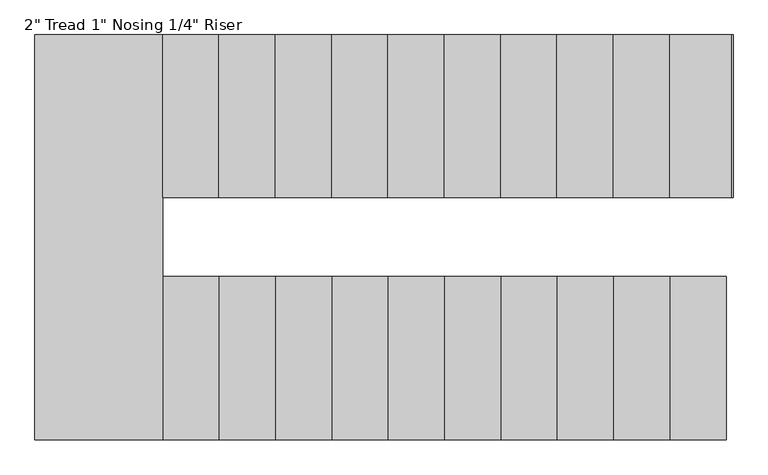
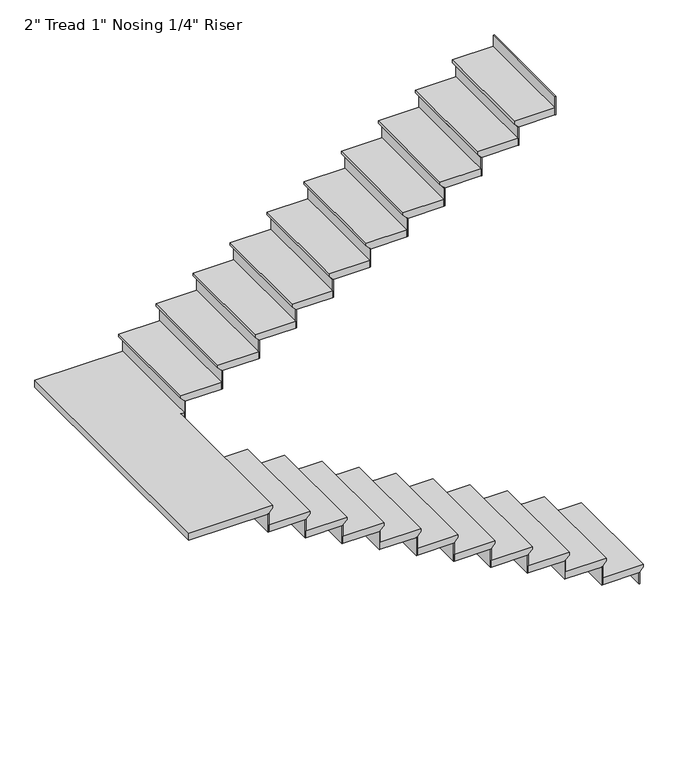
"""IFC4 building model written with IfcOpenShell, lengths in millimetres: stair flight geometry."""

from ifc_helpers import new_model, si_unit, origin, place, context, project, spatial, faceted_brep, source, transform, mapped, element, save


def stair_flight_862ef343(model_context):
    return source(origin(), model_context, "Body", "Brep", [
        faceted_brep([(-3117.2664982, -6914.3822004, 9713.7681818), (-3117.2664982, -6914.3822004, 9732.8181818), (-3117.2664982, -7650.9822004, 9732.8181818), (-3117.2664982, -7650.9822004, 9713.7681818), (-3142.6664982, -6914.3822004, 9688.3681818), (-3142.6664982, -7650.9822004, 9688.3681818), (-3396.6664982, -6914.3822004, 9732.8181818), (-3396.6664982, -7650.9822004, 9732.8181818), (-3142.6664982, -7650.9822004, 9682.0181818), (-3396.6664982, -7650.9822004, 9682.0181818), (-3396.6664982, -6914.3822004, 9682.0181818), (-3142.6664982, -6914.3822004, 9682.0181818)], [[[0, 1, 2, 3]], [[4, 0, 3, 5]], [[2, 1, 6, 7]], [[8, 9, 10, 11]], [[2, 7, 9, 8, 5, 3]], [[8, 11, 4, 5]], [[6, 1, 0, 4, 11, 10]], [[7, 6, 10, 9]]]),
        faceted_brep([(-3142.6664982, -6914.3822004, 9682.0181818), (-3142.6664982, -6914.3822004, 9601.2), (-3149.0164982, -6914.3822004, 9601.2), (-3149.0164982, -6914.3822004, 9682.0181818), (-3142.6664982, -7650.9822004, 9682.0181818), (-3149.0164982, -7650.9822004, 9682.0181818), (-3149.0164982, -7650.9822004, 9601.2), (-3142.6664982, -7650.9822004, 9601.2)], [[[0, 1, 2, 3]], [[4, 5, 6, 7]], [[1, 0, 4, 7]], [[2, 1, 7, 6]], [[3, 2, 6, 5]], [[0, 3, 5, 4]]]),
        faceted_brep([(-3396.6664982, -6914.3822004, 9813.6363636), (-3396.6664982, -6914.3822004, 9682.0181818), (-3403.0164982, -6914.3822004, 9682.0181818), (-3403.0164982, -6914.3822004, 9813.6363636), (-3396.6664982, -7650.9822004, 9813.6363636), (-3403.0164982, -7650.9822004, 9813.6363636), (-3403.0164982, -7650.9822004, 9682.0181818), (-3396.6664982, -7650.9822004, 9682.0181818)], [[[0, 1, 2, 3]], [[4, 5, 6, 7]], [[1, 0, 4, 7]], [[2, 1, 7, 6]], [[3, 2, 6, 5]], [[0, 3, 5, 4]]]),
        faceted_brep([(-3371.2664982, -7650.9822004, 9864.4363636), (-3371.2664982, -6914.3822004, 9864.4363636), (-3650.6664982, -6914.3822004, 9864.4363636), (-3650.6664982, -7650.9822004, 9864.4363636), (-3396.6664982, -7650.9822004, 9813.6363636), (-3650.6664982, -7650.9822004, 9813.6363636), (-3650.6664982, -6914.3822004, 9813.6363636), (-3396.6664982, -6914.3822004, 9813.6363636), (-3396.6664982, -7650.9822004, 9819.9863636), (-3371.2664982, -7650.9822004, 9845.3863636), (-3396.6664982, -6914.3822004, 9819.9863636), (-3371.2664982, -6914.3822004, 9845.3863636)], [[[0, 1, 2, 3]], [[4, 5, 6, 7]], [[0, 3, 5, 4, 8, 9]], [[4, 7, 10, 8]], [[2, 1, 11, 10, 7, 6]], [[3, 2, 6, 5]], [[11, 1, 0, 9]], [[10, 11, 9, 8]]]),
        faceted_brep([(-3650.6664982, -6914.3822004, 9945.2545455), (-3650.6664982, -6914.3822004, 9813.6363636), (-3657.0164982, -6914.3822004, 9813.6363636), (-3657.0164982, -6914.3822004, 9945.2545455), (-3650.6664982, -7650.9822004, 9945.2545455), (-3657.0164982, -7650.9822004, 9945.2545455), (-3657.0164982, -7650.9822004, 9813.6363636), (-3650.6664982, -7650.9822004, 9813.6363636)], [[[0, 1, 2, 3]], [[4, 5, 6, 7]], [[1, 0, 4, 7]], [[2, 1, 7, 6]], [[3, 2, 6, 5]], [[0, 3, 5, 4]]]),
        faceted_brep([(-3625.2664982, -7650.9822004, 9996.0545455), (-3625.2664982, -6914.3822004, 9996.0545455), (-3904.6664982, -6914.3822004, 9996.0545455), (-3904.6664982, -7650.9822004, 9996.0545455), (-3650.6664982, -7650.9822004, 9945.2545455), (-3904.6664982, -7650.9822004, 9945.2545455), (-3904.6664982, -6914.3822004, 9945.2545455), (-3650.6664982, -6914.3822004, 9945.2545455), (-3650.6664982, -7650.9822004, 9951.6045455), (-3625.2664982, -7650.9822004, 9977.0045455), (-3650.6664982, -6914.3822004, 9951.6045455), (-3625.2664982, -6914.3822004, 9977.0045455)], [[[0, 1, 2, 3]], [[4, 5, 6, 7]], [[0, 3, 5, 4, 8, 9]], [[4, 7, 10, 8]], [[2, 1, 11, 10, 7, 6]], [[3, 2, 6, 5]], [[11, 1, 0, 9]], [[10, 11, 9, 8]]]),
        faceted_brep([(-3904.6664982, -6914.3822004, 10076.8727273), (-3904.6664982, -6914.3822004, 9945.2545455), (-3911.0164982, -6914.3822004, 9945.2545455), (-3911.0164982, -6914.3822004, 10076.8727273), (-3904.6664982, -7650.9822004, 10076.8727273), (-3911.0164982, -7650.9822004, 10076.8727273), (-3911.0164982, -7650.9822004, 9945.2545455), (-3904.6664982, -7650.9822004, 9945.2545455)], [[[0, 1, 2, 3]], [[4, 5, 6, 7]], [[1, 0, 4, 7]], [[2, 1, 7, 6]], [[3, 2, 6, 5]], [[0, 3, 5, 4]]]),
        faceted_brep([(-3879.2664982, -7650.9822004, 10127.6727273), (-3879.2664982, -6914.3822004, 10127.6727273), (-4158.6664982, -6914.3822004, 10127.6727273), (-4158.6664982, -7650.9822004, 10127.6727273), (-3904.6664982, -7650.9822004, 10076.8727273), (-4158.6664982, -7650.9822004, 10076.8727273), (-4158.6664982, -6914.3822004, 10076.8727273), (-3904.6664982, -6914.3822004, 10076.8727273), (-3904.6664982, -7650.9822004, 10083.2227273), (-3879.2664982, -7650.9822004, 10108.6227273), (-3904.6664982, -6914.3822004, 10083.2227273), (-3879.2664982, -6914.3822004, 10108.6227273)], [[[0, 1, 2, 3]], [[4, 5, 6, 7]], [[0, 3, 5, 4, 8, 9]], [[4, 7, 10, 8]], [[2, 1, 11, 10, 7, 6]], [[3, 2, 6, 5]], [[11, 1, 0, 9]], [[10, 11, 9, 8]]]),
        faceted_brep([(-4158.6664982, -6914.3822004, 10208.4909091), (-4158.6664982, -6914.3822004, 10076.8727273), (-4165.0164982, -6914.3822004, 10076.8727273), (-4165.0164982, -6914.3822004, 10208.4909091), (-4158.6664982, -7650.9822004, 10208.4909091), (-4165.0164982, -7650.9822004, 10208.4909091), (-4165.0164982, -7650.9822004, 10076.8727273), (-4158.6664982, -7650.9822004, 10076.8727273)], [[[0, 1, 2, 3]], [[4, 5, 6, 7]], [[1, 0, 4, 7]], [[2, 1, 7, 6]], [[3, 2, 6, 5]], [[0, 3, 5, 4]]]),
        faceted_brep([(-4133.2664982, -7650.9822004, 10259.2909091), (-4133.2664982, -6914.3822004, 10259.2909091), (-4412.6664982, -6914.3822004, 10259.2909091), (-4412.6664982, -7650.9822004, 10259.2909091), (-4158.6664982, -7650.9822004, 10208.4909091), (-4412.6664982, -7650.9822004, 10208.4909091), (-4412.6664982, -6914.3822004, 10208.4909091), (-4158.6664982, -6914.3822004, 10208.4909091), (-4158.6664982, -7650.9822004, 10214.8409091), (-4133.2664982, -7650.9822004, 10240.2409091), (-4158.6664982, -6914.3822004, 10214.8409091), (-4133.2664982, -6914.3822004, 10240.2409091)], [[[0, 1, 2, 3]], [[4, 5, 6, 7]], [[0, 3, 5, 4, 8, 9]], [[4, 7, 10, 8]], [[2, 1, 11, 10, 7, 6]], [[3, 2, 6, 5]], [[11, 1, 0, 9]], [[10, 11, 9, 8]]]),
        faceted_brep([(-4412.6664982, -6914.3822004, 10340.1090909), (-4412.6664982, -6914.3822004, 10208.4909091), (-4419.0164982, -6914.3822004, 10208.4909091), (-4419.0164982, -6914.3822004, 10340.1090909), (-4412.6664982, -7650.9822004, 10340.1090909), (-4419.0164982, -7650.9822004, 10340.1090909), (-4419.0164982, -7650.9822004, 10208.4909091), (-4412.6664982, -7650.9822004, 10208.4909091)], [[[0, 1, 2, 3]], [[4, 5, 6, 7]], [[1, 0, 4, 7]], [[2, 1, 7, 6]], [[3, 2, 6, 5]], [[0, 3, 5, 4]]]),
        faceted_brep([(-4387.2664982, -7650.9822004, 10390.9090909), (-4387.2664982, -6914.3822004, 10390.9090909), (-4666.6664982, -6914.3822004, 10390.9090909), (-4666.6664982, -7650.9822004, 10390.9090909), (-4412.6664982, -7650.9822004, 10340.1090909), (-4666.6664982, -7650.9822004, 10340.1090909), (-4666.6664982, -6914.3822004, 10340.1090909), (-4412.6664982, -6914.3822004, 10340.1090909), (-4412.6664982, -7650.9822004, 10346.4590909), (-4387.2664982, -7650.9822004, 10371.8590909), (-4412.6664982, -6914.3822004, 10346.4590909), (-4387.2664982, -6914.3822004, 10371.8590909)], [[[0, 1, 2, 3]], [[4, 5, 6, 7]], [[0, 3, 5, 4, 8, 9]], [[4, 7, 10, 8]], [[2, 1, 11, 10, 7, 6]], [[3, 2, 6, 5]], [[11, 1, 0, 9]], [[10, 11, 9, 8]]]),
        faceted_brep([(-4666.6664982, -6914.3822004, 10471.7272727), (-4666.6664982, -6914.3822004, 10340.1090909), (-4673.0164982, -6914.3822004, 10340.1090909), (-4673.0164982, -6914.3822004, 10471.7272727), (-4666.6664982, -7650.9822004, 10471.7272727), (-4673.0164982, -7650.9822004, 10471.7272727), (-4673.0164982, -7650.9822004, 10340.1090909), (-4666.6664982, -7650.9822004, 10340.1090909)], [[[0, 1, 2, 3]], [[4, 5, 6, 7]], [[1, 0, 4, 7]], [[2, 1, 7, 6]], [[3, 2, 6, 5]], [[0, 3, 5, 4]]]),
        faceted_brep([(-4641.2664982, -7650.9822004, 10522.5272727), (-4641.2664982, -6914.3822004, 10522.5272727), (-4920.6664982, -6914.3822004, 10522.5272727), (-4920.6664982, -7650.9822004, 10522.5272727), (-4666.6664982, -7650.9822004, 10471.7272727), (-4920.6664982, -7650.9822004, 10471.7272727), (-4920.6664982, -6914.3822004, 10471.7272727), (-4666.6664982, -6914.3822004, 10471.7272727), (-4666.6664982, -7650.9822004, 10478.0772727), (-4641.2664982, -7650.9822004, 10503.4772727), (-4666.6664982, -6914.3822004, 10478.0772727), (-4641.2664982, -6914.3822004, 10503.4772727)], [[[0, 1, 2, 3]], [[4, 5, 6, 7]], [[0, 3, 5, 4, 8, 9]], [[4, 7, 10, 8]], [[2, 1, 11, 10, 7, 6]], [[3, 2, 6, 5]], [[11, 1, 0, 9]], [[10, 11, 9, 8]]]),
        faceted_brep([(-4920.6664982, -6914.3822004, 10603.3454545), (-4920.6664982, -6914.3822004, 10471.7272727), (-4927.0164982, -6914.3822004, 10471.7272727), (-4927.0164982, -6914.3822004, 10603.3454545), (-4920.6664982, -7650.9822004, 10603.3454545), (-4927.0164982, -7650.9822004, 10603.3454545), (-4927.0164982, -7650.9822004, 10471.7272727), (-4920.6664982, -7650.9822004, 10471.7272727)], [[[0, 1, 2, 3]], [[4, 5, 6, 7]], [[1, 0, 4, 7]], [[2, 1, 7, 6]], [[3, 2, 6, 5]], [[0, 3, 5, 4]]]),
        faceted_brep([(-4895.2664982, -7650.9822004, 10654.1454545), (-4895.2664982, -6914.3822004, 10654.1454545), (-5174.6664982, -6914.3822004, 10654.1454545), (-5174.6664982, -7650.9822004, 10654.1454545), (-4920.6664982, -7650.9822004, 10603.3454545), (-5174.6664982, -7650.9822004, 10603.3454545), (-5174.6664982, -6914.3822004, 10603.3454545), (-4920.6664982, -6914.3822004, 10603.3454545), (-4920.6664982, -7650.9822004, 10609.6954545), (-4895.2664982, -7650.9822004, 10635.0954545), (-4920.6664982, -6914.3822004, 10609.6954545), (-4895.2664982, -6914.3822004, 10635.0954545)], [[[0, 1, 2, 3]], [[4, 5, 6, 7]], [[0, 3, 5, 4, 8, 9]], [[4, 7, 10, 8]], [[2, 1, 11, 10, 7, 6]], [[3, 2, 6, 5]], [[11, 1, 0, 9]], [[10, 11, 9, 8]]]),
        faceted_brep([(-5174.6664982, -6914.3822004, 10734.9636364), (-5174.6664982, -6914.3822004, 10603.3454545), (-5181.0164982, -6914.3822004, 10603.3454545), (-5181.0164982, -6914.3822004, 10734.9636364), (-5174.6664982, -7650.9822004, 10734.9636364), (-5181.0164982, -7650.9822004, 10734.9636364), (-5181.0164982, -7650.9822004, 10603.3454545), (-5174.6664982, -7650.9822004, 10603.3454545)], [[[0, 1, 2, 3]], [[4, 5, 6, 7]], [[1, 0, 4, 7]], [[2, 1, 7, 6]], [[3, 2, 6, 5]], [[0, 3, 5, 4]]]),
        faceted_brep([(-5149.2664982, -7650.9822004, 10785.7636364), (-5149.2664982, -6914.3822004, 10785.7636364), (-5428.6664982, -6914.3822004, 10785.7636364), (-5428.6664982, -7650.9822004, 10785.7636364), (-5174.6664982, -7650.9822004, 10734.9636364), (-5428.6664982, -7650.9822004, 10734.9636364), (-5428.6664982, -6914.3822004, 10734.9636364), (-5174.6664982, -6914.3822004, 10734.9636364), (-5174.6664982, -7650.9822004, 10741.3136364), (-5149.2664982, -7650.9822004, 10766.7136364), (-5174.6664982, -6914.3822004, 10741.3136364), (-5149.2664982, -6914.3822004, 10766.7136364)], [[[0, 1, 2, 3]], [[4, 5, 6, 7]], [[0, 3, 5, 4, 8, 9]], [[4, 7, 10, 8]], [[2, 1, 11, 10, 7, 6]], [[3, 2, 6, 5]], [[11, 1, 0, 9]], [[10, 11, 9, 8]]]),
        faceted_brep([(-5428.6664982, -6914.3822004, 10866.5818182), (-5428.6664982, -6914.3822004, 10734.9636364), (-5435.0164982, -6914.3822004, 10734.9636364), (-5435.0164982, -6914.3822004, 10866.5818182), (-5428.6664982, -7650.9822004, 10866.5818182), (-5435.0164982, -7650.9822004, 10866.5818182), (-5435.0164982, -7650.9822004, 10734.9636364), (-5428.6664982, -7650.9822004, 10734.9636364)], [[[0, 1, 2, 3]], [[4, 5, 6, 7]], [[1, 0, 4, 7]], [[2, 1, 7, 6]], [[3, 2, 6, 5]], [[0, 3, 5, 4]]]),
        faceted_brep([(-5403.2664982, -7650.9822004, 10917.3818182), (-5403.2664982, -6914.3822004, 10917.3818182), (-5682.6664982, -6914.3822004, 10917.3818182), (-5682.6664982, -7650.9822004, 10917.3818182), (-5428.6664982, -7650.9822004, 10866.5818182), (-5682.6664982, -7650.9822004, 10866.5818182), (-5682.6664982, -6914.3822004, 10866.5818182), (-5428.6664982, -6914.3822004, 10866.5818182), (-5428.6664982, -7650.9822004, 10872.9318182), (-5403.2664982, -7650.9822004, 10898.3318182), (-5428.6664982, -6914.3822004, 10872.9318182), (-5403.2664982, -6914.3822004, 10898.3318182)], [[[0, 1, 2, 3]], [[4, 5, 6, 7]], [[0, 3, 5, 4, 8, 9]], [[4, 7, 10, 8]], [[2, 1, 11, 10, 7, 6]], [[3, 2, 6, 5]], [[11, 1, 0, 9]], [[10, 11, 9, 8]]]),
        faceted_brep([(-5682.6664982, -6914.3822004, 10998.2), (-5682.6664982, -6914.3822004, 10866.5818182), (-5689.0164982, -6914.3822004, 10866.5818182), (-5689.0164982, -6914.3822004, 10998.2), (-5682.6664982, -7650.9822004, 10998.2), (-5689.0164982, -7650.9822004, 10998.2), (-5689.0164982, -7650.9822004, 10866.5818182), (-5682.6664982, -7650.9822004, 10866.5818182)], [[[0, 1, 2, 3]], [[4, 5, 6, 7]], [[1, 0, 4, 7]], [[2, 1, 7, 6]], [[3, 2, 6, 5]], [[0, 3, 5, 4]]]),
        faceted_brep([(-5631.8664982, -5824.7082131, 11049.0), (-6232.5131972, -5824.7082131, 11049.0), (-6232.5131972, -7650.9822004, 11049.0), (-5657.2664982, -7650.9822004, 11049.0), (-5657.2664982, -6558.7822004, 11049.0), (-5631.8664982, -6558.7822004, 11049.0), (-6232.5131972, -5824.7082131, 10998.2), (-5631.8664982, -5824.7082131, 10998.2), (-5631.8664982, -6558.7822004, 10998.2), (-5657.2664982, -6558.7822004, 10998.2), (-5657.2664982, -6914.3822004, 10998.2), (-5682.6664982, -6914.3822004, 10998.2), (-5682.6664982, -7650.9822004, 10998.2), (-6232.5131972, -7650.9822004, 10998.2), (-5682.6664982, -6914.3822004, 11004.55), (-5682.6664982, -7650.9822004, 11004.55), (-5657.2664982, -7650.9822004, 11029.95), (-5657.2664982, -6914.3822004, 11029.95)], [[[0, 1, 2, 3, 4, 5]], [[6, 7, 8, 9, 10, 11, 12, 13]], [[1, 0, 7, 6]], [[2, 1, 6, 13]], [[12, 11, 14, 15]], [[4, 3, 16, 17, 10, 9]], [[5, 4, 9, 8]], [[0, 5, 8, 7]], [[16, 15, 14, 17]], [[3, 2, 13, 12, 15, 16]], [[11, 10, 17, 14]]]),
        faceted_brep([(-5631.8664982, -6558.7822004, 11129.8181818), (-5631.8664982, -6558.7822004, 10998.2), (-5625.5164982, -6558.7822004, 10998.2), (-5625.5164982, -6558.7822004, 11129.8181818), (-5631.8664982, -5824.7082131, 11129.8181818), (-5625.5164982, -5824.7082131, 11129.8181818), (-5625.5164982, -5824.7082131, 10998.2), (-5631.8664982, -5824.7082131, 10998.2)], [[[0, 1, 2, 3]], [[4, 5, 6, 7]], [[1, 0, 4, 7]], [[2, 1, 7, 6]], [[3, 2, 6, 5]], [[0, 3, 5, 4]]]),
        faceted_brep([(-5657.2664982, -5824.7082131, 11180.6181818), (-5657.2664982, -6558.7822004, 11180.6181818), (-5377.8664982, -6558.7822004, 11180.6181818), (-5377.8664982, -5824.7082131, 11180.6181818), (-5631.8664982, -5824.7082131, 11129.8181818), (-5377.8664982, -5824.7082131, 11129.8181818), (-5377.8664982, -6558.7822004, 11129.8181818), (-5631.8664982, -6558.7822004, 11129.8181818), (-5631.8664982, -5824.7082131, 11136.1681818), (-5657.2664982, -5824.7082131, 11161.5681818), (-5631.8664982, -6558.7822004, 11136.1681818), (-5657.2664982, -6558.7822004, 11161.5681818)], [[[0, 1, 2, 3]], [[4, 5, 6, 7]], [[0, 3, 5, 4, 8, 9]], [[4, 7, 10, 8]], [[2, 1, 11, 10, 7, 6]], [[3, 2, 6, 5]], [[11, 1, 0, 9]], [[10, 11, 9, 8]]]),
        faceted_brep([(-5377.8664982, -6558.7822004, 11261.4363636), (-5377.8664982, -6558.7822004, 11129.8181818), (-5371.5164982, -6558.7822004, 11129.8181818), (-5371.5164982, -6558.7822004, 11261.4363636), (-5377.8664982, -5824.7082131, 11261.4363636), (-5371.5164982, -5824.7082131, 11261.4363636), (-5371.5164982, -5824.7082131, 11129.8181818), (-5377.8664982, -5824.7082131, 11129.8181818)], [[[0, 1, 2, 3]], [[4, 5, 6, 7]], [[1, 0, 4, 7]], [[2, 1, 7, 6]], [[3, 2, 6, 5]], [[0, 3, 5, 4]]]),
        faceted_brep([(-5403.2664982, -5824.7082131, 11312.2363636), (-5403.2664982, -6558.7822004, 11312.2363636), (-5123.8664982, -6558.7822004, 11312.2363636), (-5123.8664982, -5824.7082131, 11312.2363636), (-5377.8664982, -5824.7082131, 11261.4363636), (-5123.8664982, -5824.7082131, 11261.4363636), (-5123.8664982, -6558.7822004, 11261.4363636), (-5377.8664982, -6558.7822004, 11261.4363636), (-5377.8664982, -5824.7082131, 11267.7863636), (-5403.2664982, -5824.7082131, 11293.1863636), (-5377.8664982, -6558.7822004, 11267.7863636), (-5403.2664982, -6558.7822004, 11293.1863636)], [[[0, 1, 2, 3]], [[4, 5, 6, 7]], [[0, 3, 5, 4, 8, 9]], [[4, 7, 10, 8]], [[2, 1, 11, 10, 7, 6]], [[3, 2, 6, 5]], [[11, 1, 0, 9]], [[10, 11, 9, 8]]]),
        faceted_brep([(-5123.8664982, -6558.7822004, 11393.0545455), (-5123.8664982, -6558.7822004, 11261.4363636), (-5117.5164982, -6558.7822004, 11261.4363636), (-5117.5164982, -6558.7822004, 11393.0545455), (-5123.8664982, -5824.7082131, 11393.0545455), (-5117.5164982, -5824.7082131, 11393.0545455), (-5117.5164982, -5824.7082131, 11261.4363636), (-5123.8664982, -5824.7082131, 11261.4363636)], [[[0, 1, 2, 3]], [[4, 5, 6, 7]], [[1, 0, 4, 7]], [[2, 1, 7, 6]], [[3, 2, 6, 5]], [[0, 3, 5, 4]]]),
        faceted_brep([(-5149.2664982, -5824.7082131, 11443.8545455), (-5149.2664982, -6558.7822004, 11443.8545455), (-4869.8664982, -6558.7822004, 11443.8545455), (-4869.8664982, -5824.7082131, 11443.8545455), (-5123.8664982, -5824.7082131, 11393.0545455), (-4869.8664982, -5824.7082131, 11393.0545455), (-4869.8664982, -6558.7822004, 11393.0545455), (-5123.8664982, -6558.7822004, 11393.0545455), (-5123.8664982, -5824.7082131, 11399.4045455), (-5149.2664982, -5824.7082131, 11424.8045455), (-5123.8664982, -6558.7822004, 11399.4045455), (-5149.2664982, -6558.7822004, 11424.8045455)], [[[0, 1, 2, 3]], [[4, 5, 6, 7]], [[0, 3, 5, 4, 8, 9]], [[4, 7, 10, 8]], [[2, 1, 11, 10, 7, 6]], [[3, 2, 6, 5]], [[11, 1, 0, 9]], [[10, 11, 9, 8]]]),
        faceted_brep([(-4869.8664982, -6558.7822004, 11524.6727273), (-4869.8664982, -6558.7822004, 11393.0545455), (-4863.5164982, -6558.7822004, 11393.0545455), (-4863.5164982, -6558.7822004, 11524.6727273), (-4869.8664982, -5824.7082131, 11524.6727273), (-4863.5164982, -5824.7082131, 11524.6727273), (-4863.5164982, -5824.7082131, 11393.0545455), (-4869.8664982, -5824.7082131, 11393.0545455)], [[[0, 1, 2, 3]], [[4, 5, 6, 7]], [[1, 0, 4, 7]], [[2, 1, 7, 6]], [[3, 2, 6, 5]], [[0, 3, 5, 4]]]),
        faceted_brep([(-4895.2664982, -5824.7082131, 11575.4727273), (-4895.2664982, -6558.7822004, 11575.4727273), (-4615.8664982, -6558.7822004, 11575.4727273), (-4615.8664982, -5824.7082131, 11575.4727273), (-4869.8664982, -5824.7082131, 11524.6727273), (-4615.8664982, -5824.7082131, 11524.6727273), (-4615.8664982, -6558.7822004, 11524.6727273), (-4869.8664982, -6558.7822004, 11524.6727273), (-4869.8664982, -5824.7082131, 11531.0227273), (-4895.2664982, -5824.7082131, 11556.4227273), (-4869.8664982, -6558.7822004, 11531.0227273), (-4895.2664982, -6558.7822004, 11556.4227273)], [[[0, 1, 2, 3]], [[4, 5, 6, 7]], [[0, 3, 5, 4, 8, 9]], [[4, 7, 10, 8]], [[2, 1, 11, 10, 7, 6]], [[3, 2, 6, 5]], [[11, 1, 0, 9]], [[10, 11, 9, 8]]]),
        faceted_brep([(-4615.8664982, -6558.7822004, 11656.2909091), (-4615.8664982, -6558.7822004, 11524.6727273), (-4609.5164982, -6558.7822004, 11524.6727273), (-4609.5164982, -6558.7822004, 11656.2909091), (-4615.8664982, -5824.7082131, 11656.2909091), (-4609.5164982, -5824.7082131, 11656.2909091), (-4609.5164982, -5824.7082131, 11524.6727273), (-4615.8664982, -5824.7082131, 11524.6727273)], [[[0, 1, 2, 3]], [[4, 5, 6, 7]], [[1, 0, 4, 7]], [[2, 1, 7, 6]], [[3, 2, 6, 5]], [[0, 3, 5, 4]]]),
        faceted_brep([(-4641.2664982, -5824.7082131, 11707.0909091), (-4641.2664982, -6558.7822004, 11707.0909091), (-4361.8664982, -6558.7822004, 11707.0909091), (-4361.8664982, -5824.7082131, 11707.0909091), (-4615.8664982, -5824.7082131, 11656.2909091), (-4361.8664982, -5824.7082131, 11656.2909091), (-4361.8664982, -6558.7822004, 11656.2909091), (-4615.8664982, -6558.7822004, 11656.2909091), (-4615.8664982, -5824.7082131, 11662.6409091), (-4641.2664982, -5824.7082131, 11688.0409091), (-4615.8664982, -6558.7822004, 11662.6409091), (-4641.2664982, -6558.7822004, 11688.0409091)], [[[0, 1, 2, 3]], [[4, 5, 6, 7]], [[0, 3, 5, 4, 8, 9]], [[4, 7, 10, 8]], [[2, 1, 11, 10, 7, 6]], [[3, 2, 6, 5]], [[11, 1, 0, 9]], [[10, 11, 9, 8]]]),
        faceted_brep([(-4361.8664982, -6558.7822004, 11787.9090909), (-4361.8664982, -6558.7822004, 11656.2909091), (-4355.5164982, -6558.7822004, 11656.2909091), (-4355.5164982, -6558.7822004, 11787.9090909), (-4361.8664982, -5824.7082131, 11787.9090909), (-4355.5164982, -5824.7082131, 11787.9090909), (-4355.5164982, -5824.7082131, 11656.2909091), (-4361.8664982, -5824.7082131, 11656.2909091)], [[[0, 1, 2, 3]], [[4, 5, 6, 7]], [[1, 0, 4, 7]], [[2, 1, 7, 6]], [[3, 2, 6, 5]], [[0, 3, 5, 4]]]),
        faceted_brep([(-4387.2664982, -5824.7082131, 11838.7090909), (-4387.2664982, -6558.7822004, 11838.7090909), (-4107.8664982, -6558.7822004, 11838.7090909), (-4107.8664982, -5824.7082131, 11838.7090909), (-4361.8664982, -5824.7082131, 11787.9090909), (-4107.8664982, -5824.7082131, 11787.9090909), (-4107.8664982, -6558.7822004, 11787.9090909), (-4361.8664982, -6558.7822004, 11787.9090909), (-4361.8664982, -5824.7082131, 11794.2590909), (-4387.2664982, -5824.7082131, 11819.6590909), (-4361.8664982, -6558.7822004, 11794.2590909), (-4387.2664982, -6558.7822004, 11819.6590909)], [[[0, 1, 2, 3]], [[4, 5, 6, 7]], [[0, 3, 5, 4, 8, 9]], [[4, 7, 10, 8]], [[2, 1, 11, 10, 7, 6]], [[3, 2, 6, 5]], [[11, 1, 0, 9]], [[10, 11, 9, 8]]]),
        faceted_brep([(-4107.8664982, -6558.7822004, 11919.5272727), (-4107.8664982, -6558.7822004, 11787.9090909), (-4101.5164982, -6558.7822004, 11787.9090909), (-4101.5164982, -6558.7822004, 11919.5272727), (-4107.8664982, -5824.7082131, 11919.5272727), (-4101.5164982, -5824.7082131, 11919.5272727), (-4101.5164982, -5824.7082131, 11787.9090909), (-4107.8664982, -5824.7082131, 11787.9090909)], [[[0, 1, 2, 3]], [[4, 5, 6, 7]], [[1, 0, 4, 7]], [[2, 1, 7, 6]], [[3, 2, 6, 5]], [[0, 3, 5, 4]]]),
        faceted_brep([(-4133.2664982, -5824.7082131, 11970.3272727), (-4133.2664982, -6558.7822004, 11970.3272727), (-3853.8664982, -6558.7822004, 11970.3272727), (-3853.8664982, -5824.7082131, 11970.3272727), (-4107.8664982, -5824.7082131, 11919.5272727), (-3853.8664982, -5824.7082131, 11919.5272727), (-3853.8664982, -6558.7822004, 11919.5272727), (-4107.8664982, -6558.7822004, 11919.5272727), (-4107.8664982, -5824.7082131, 11925.8772727), (-4133.2664982, -5824.7082131, 11951.2772727), (-4107.8664982, -6558.7822004, 11925.8772727), (-4133.2664982, -6558.7822004, 11951.2772727)], [[[0, 1, 2, 3]], [[4, 5, 6, 7]], [[0, 3, 5, 4, 8, 9]], [[4, 7, 10, 8]], [[2, 1, 11, 10, 7, 6]], [[3, 2, 6, 5]], [[11, 1, 0, 9]], [[10, 11, 9, 8]]]),
        faceted_brep([(-3853.8664982, -6558.7822004, 12051.1454545), (-3853.8664982, -6558.7822004, 11919.5272727), (-3847.5164982, -6558.7822004, 11919.5272727), (-3847.5164982, -6558.7822004, 12051.1454545), (-3853.8664982, -5824.7082131, 12051.1454545), (-3847.5164982, -5824.7082131, 12051.1454545), (-3847.5164982, -5824.7082131, 11919.5272727), (-3853.8664982, -5824.7082131, 11919.5272727)], [[[0, 1, 2, 3]], [[4, 5, 6, 7]], [[1, 0, 4, 7]], [[2, 1, 7, 6]], [[3, 2, 6, 5]], [[0, 3, 5, 4]]]),
        faceted_brep([(-3879.2664982, -5824.7082131, 12101.9454545), (-3879.2664982, -6558.7822004, 12101.9454545), (-3599.8664982, -6558.7822004, 12101.9454545), (-3599.8664982, -5824.7082131, 12101.9454545), (-3853.8664982, -5824.7082131, 12051.1454545), (-3599.8664982, -5824.7082131, 12051.1454545), (-3599.8664982, -6558.7822004, 12051.1454545), (-3853.8664982, -6558.7822004, 12051.1454545), (-3853.8664982, -5824.7082131, 12057.4954545), (-3879.2664982, -5824.7082131, 12082.8954545), (-3853.8664982, -6558.7822004, 12057.4954545), (-3879.2664982, -6558.7822004, 12082.8954545)], [[[0, 1, 2, 3]], [[4, 5, 6, 7]], [[0, 3, 5, 4, 8, 9]], [[4, 7, 10, 8]], [[2, 1, 11, 10, 7, 6]], [[3, 2, 6, 5]], [[11, 1, 0, 9]], [[10, 11, 9, 8]]]),
        faceted_brep([(-3599.8664982, -6558.7822004, 12182.7636364), (-3599.8664982, -6558.7822004, 12051.1454545), (-3593.5164982, -6558.7822004, 12051.1454545), (-3593.5164982, -6558.7822004, 12182.7636364), (-3599.8664982, -5824.7082131, 12182.7636364), (-3593.5164982, -5824.7082131, 12182.7636364), (-3593.5164982, -5824.7082131, 12051.1454545), (-3599.8664982, -5824.7082131, 12051.1454545)], [[[0, 1, 2, 3]], [[4, 5, 6, 7]], [[1, 0, 4, 7]], [[2, 1, 7, 6]], [[3, 2, 6, 5]], [[0, 3, 5, 4]]]),
        faceted_brep([(-3625.2664982, -5824.7082131, 12233.5636364), (-3625.2664982, -6558.7822004, 12233.5636364), (-3345.8664982, -6558.7822004, 12233.5636364), (-3345.8664982, -5824.7082131, 12233.5636364), (-3599.8664982, -5824.7082131, 12182.7636364), (-3345.8664982, -5824.7082131, 12182.7636364), (-3345.8664982, -6558.7822004, 12182.7636364), (-3599.8664982, -6558.7822004, 12182.7636364), (-3599.8664982, -5824.7082131, 12189.1136364), (-3625.2664982, -5824.7082131, 12214.5136364), (-3599.8664982, -6558.7822004, 12189.1136364), (-3625.2664982, -6558.7822004, 12214.5136364)], [[[0, 1, 2, 3]], [[4, 5, 6, 7]], [[0, 3, 5, 4, 8, 9]], [[4, 7, 10, 8]], [[2, 1, 11, 10, 7, 6]], [[3, 2, 6, 5]], [[11, 1, 0, 9]], [[10, 11, 9, 8]]]),
        faceted_brep([(-3345.8664982, -6558.7822004, 12314.3818182), (-3345.8664982, -6558.7822004, 12182.7636364), (-3339.5164982, -6558.7822004, 12182.7636364), (-3339.5164982, -6558.7822004, 12314.3818182), (-3345.8664982, -5824.7082131, 12314.3818182), (-3339.5164982, -5824.7082131, 12314.3818182), (-3339.5164982, -5824.7082131, 12182.7636364), (-3345.8664982, -5824.7082131, 12182.7636364)], [[[0, 1, 2, 3]], [[4, 5, 6, 7]], [[1, 0, 4, 7]], [[2, 1, 7, 6]], [[3, 2, 6, 5]], [[0, 3, 5, 4]]]),
        faceted_brep([(-3091.8664982, -6558.7822004, 12446.0), (-3091.8664982, -6558.7822004, 12314.3818182), (-3085.5164982, -6558.7822004, 12314.3818182), (-3085.5164982, -6558.7822004, 12446.0), (-3091.8664982, -5824.7082131, 12446.0), (-3085.5164982, -5824.7082131, 12446.0), (-3085.5164982, -5824.7082131, 12314.3818182), (-3091.8664982, -5824.7082131, 12314.3818182)], [[[0, 1, 2, 3]], [[4, 5, 6, 7]], [[1, 0, 4, 7]], [[2, 1, 7, 6]], [[3, 2, 6, 5]], [[0, 3, 5, 4]]]),
        faceted_brep([(-3371.2664982, -5824.7082131, 12365.1818182), (-3371.2664982, -6558.7822004, 12365.1818182), (-3091.8664982, -6558.7822004, 12365.1818182), (-3091.8664982, -5824.7082131, 12365.1818182), (-3345.8664982, -5824.7082131, 12314.3818182), (-3091.8664982, -5824.7082131, 12314.3818182), (-3091.8664982, -6558.7822004, 12314.3818182), (-3345.8664982, -6558.7822004, 12314.3818182), (-3345.8664982, -5824.7082131, 12320.7318182), (-3371.2664982, -5824.7082131, 12346.1318182), (-3345.8664982, -6558.7822004, 12320.7318182), (-3371.2664982, -6558.7822004, 12346.1318182)], [[[0, 1, 2, 3]], [[4, 5, 6, 7]], [[0, 3, 5, 4, 8, 9]], [[4, 7, 10, 8]], [[2, 1, 11, 10, 7, 6]], [[3, 2, 6, 5]], [[11, 1, 0, 9]], [[10, 11, 9, 8]]]),
    ])


if __name__ == "__main__":
    model = new_model("IFC4")
    model_context = context("Model", 3, world=origin())
    ifc_project = project(units=[si_unit("LENGTHUNIT", "METRE", prefix="MILLI")], contexts=[model_context])
    site = spatial("IfcSite", under=ifc_project)
    building = spatial("IfcBuilding", under=site)
    placement = place(None, origin())
    stair_flight_shape = stair_flight_862ef343(model_context)
    element("IfcStairFlight", 1, ObjectType="2\" Tread 1\" Nosing 1/4\" Riser", at=placement, inside=building, context=model_context, shape_type="MappedRepresentation", body=[
        mapped(stair_flight_shape, transform((0.0, 0.0, 0.0), x_axis=(1.0, 0.0, 0.0), y_axis=(0.0, 1.0, 0.0), z_axis=(0.0, 0.0, 1.0))),
    ])
    save(model, "model.ifc")
